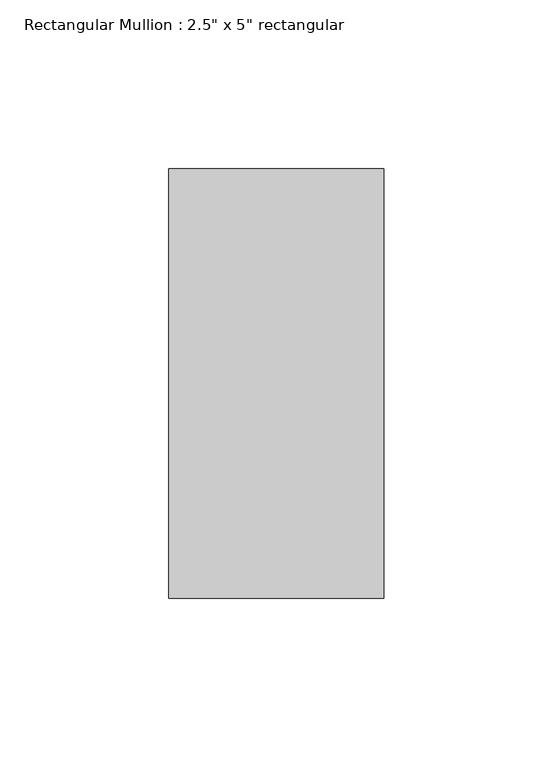
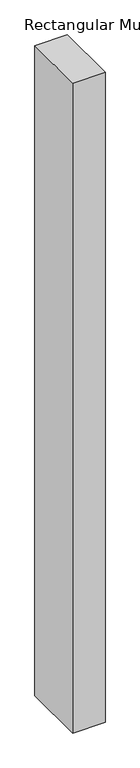
"""IFC4 building model written with IfcOpenShell, lengths in millimetres: member geometry."""

from ifc_helpers import new_model, si_unit, frame, origin, place, context, project, spatial, polyline, outline, extrude, source, transform, mapped, element, save


def member_69204bcc(model_context):
    return source(origin(), model_context, "Body", "SweptSolid", [
        extrude(outline(polyline([(0.0, 63.5), (0.0, -63.5), (-63.5, -63.5), (-63.5, 63.5), (0.0, 63.5)])), frame((0.0, 0.0, -1339.85), z_axis=(0.0, 0.0, 1.0), x_axis=(1.0, 0.0, 0.0)), (0.0, 0.0, 1.0), 1339.85),
    ])


if __name__ == "__main__":
    model = new_model("IFC4")
    model_context = context("Model", 3, world=origin())
    ifc_project = project(units=[si_unit("LENGTHUNIT", "METRE", prefix="MILLI")], contexts=[model_context])
    site = spatial("IfcSite", under=ifc_project)
    building = spatial("IfcBuilding", under=site)
    placement = place(None, origin())
    member_shape = member_69204bcc(model_context)
    element("IfcMember", 1, ObjectType="Rectangular Mullion : 2.5\" x 5\" rectangular", at=placement, inside=building, context=model_context, shape_type="MappedRepresentation", body=[
        mapped(member_shape, transform((0.0, 0.0, 0.0), x_axis=(1.0, 0.0, 0.0), y_axis=(0.0, 1.0, 0.0), z_axis=(0.0, 0.0, 1.0))),
    ])
    save(model, "model.ifc")

# Revit data of these elements
# Type "Rectangular Mullion : 2.5\" x 5\" rectangular"
#   built-in parameter 1007304 = 0.416667 (stored number, unit not read)
#   built-in parameter 1007301 = 0.104167 (stored number, unit not read)
#   built-in parameter 1007300 = 0.104167 (stored number, unit not read)
# Element 1 (IfcMember, "Rectangular Mullion : 2.5\" x 5\" rectangular")
#   Materials on its faces: "Aluminum"
# Materials
#   "Aluminum": class "Metal", colour RGB 247 247 247, transparency 0, Description = "Aluminum 6061", Cost = 0
